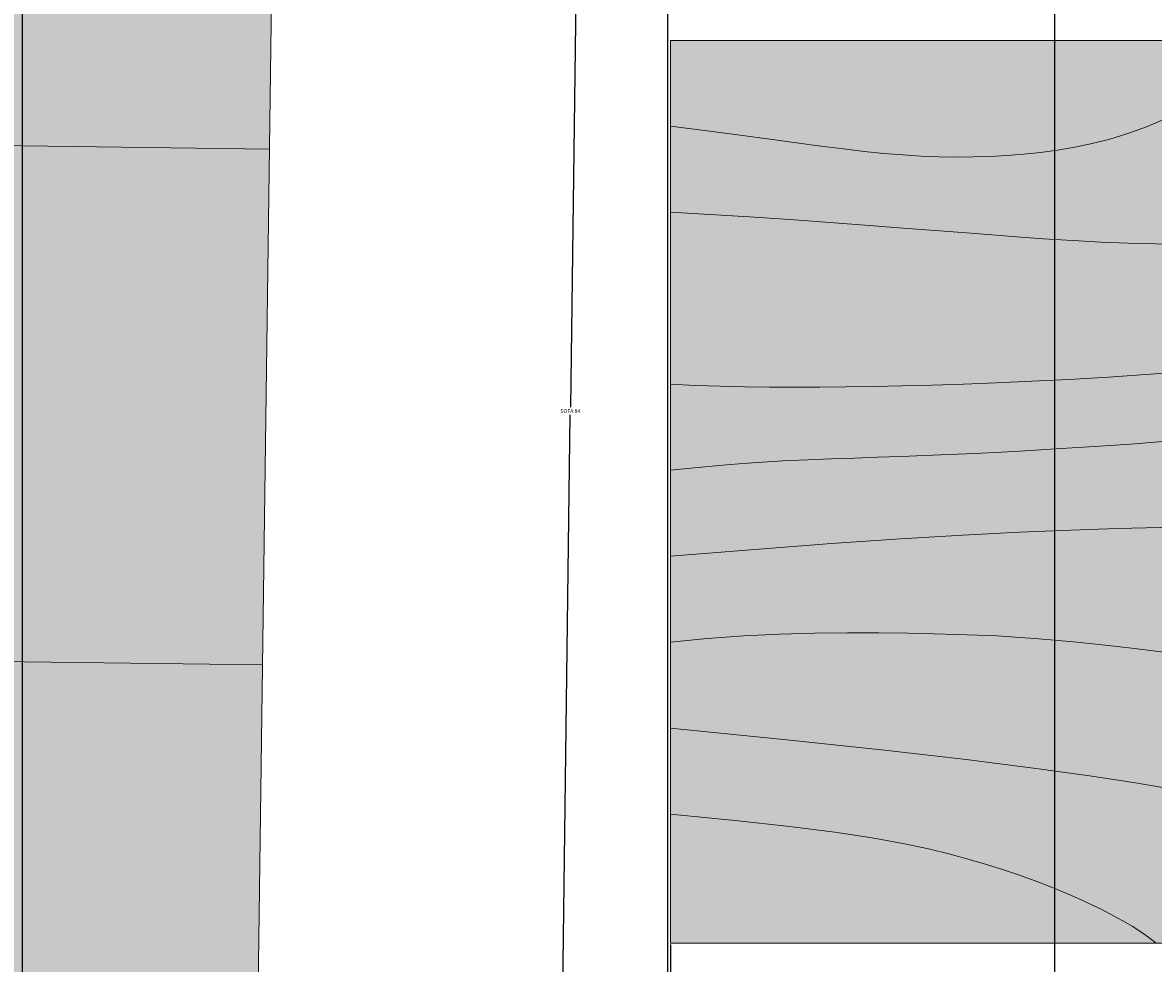
# Model space of a CAD drawing. Units: inches. Extents: x 1567 to 1964, y 1813 to 2447.
# Tile 9 of 28: x 1630 to 1683, y 2180 to 2224. Entities that reach past the tile are written whole.
import ezdxf

# ---------------------------------------------------------------- set-up
doc = ezdxf.new("R2010")
doc.units = ezdxf.units.IN
doc.layers.add('A-ANNO-DIMS', color=2, linetype='Continuous', lineweight=18)
doc.layers.add('A-FURN', color=8, linetype='Continuous', lineweight=18)
doc.layers.add('A-FURN-PATT', color=252, linetype='Continuous', lineweight=13, true_color=0x939598)
doc.styles.get("Standard").update_dxf_attribs({"font": 'arial.ttf'})
doc.dimstyles.get("Standard").update_dxf_attribs({"dimtxt": 0.18, "dimasz": 0.18, "dimexe": 0.18, "dimexo": 0.0625, "dimgap": 0.09, "dimtad": 0, "dimtih": 1, "dimtoh": 1, "dimdec": 4, "dimzin": 0, "dimdsep": 46, "dimtxsty": 'Standard', "dimcen": 0.09, "dimadec": 0, "dimazin": 0, "dimtfac": 1, "dimtdec": 4, "dimtofl": 0, "dimtmove": 0, "dimatfit": 3, "dimfxl": 1, "dimtolj": 1, "dimtzin": 0, "dimarcsym": 0})

# ---------------------------------------------------------------- blocks, each defined once
blk = doc.blocks.new('Table - Square Woodgrain 42 x 42 in.')
blk.add_line((0, -42), (42, -42))
for points in [[(0, -4), (1.704, -4.2172), (3.2358, -4.4188), (4.615, -4.604), (5.8615, -4.7721), (6.9951, -4.9224), (8.0357, -5.0541), (9.0031, -5.1667), (9.9171, -5.2594), (10.7951, -5.3316), (11.6445, -5.3836), (12.4702, -5.4157), (13.277, -5.4283), (14.0698, -5.4217), (14.8535, -5.3964), (15.6331, -5.3526), (16.4133, -5.2908), (17.1986, -5.2103), (17.9913, -5.1062), (18.793, -4.9727), (19.6056, -4.8038), (20.4307, -4.5937), (21.2701, -4.3365), (22.1256, -4.0262), (22.9989, -3.6571), (23.888, -3.2272), (24.7756, -2.7516), (25.6408, -2.2491), (26.4624, -1.7387), (27.2195, -1.2395), (27.891, -0.7703), (28.456, -0.3501), (28.8934, 0.002)], [(0, -42), (0, 0), (42, 0), (42, -42)], [(0, -8), (1.8203, -8.1001), (3.6741, -8.2149), (5.5411, -8.3408), (7.4011, -8.4741), (9.2339, -8.6112), (11.0193, -8.7484), (12.7371, -8.8821), (14.3671, -9.0086), (15.8954, -9.1246), (17.3337, -9.2278), (18.6997, -9.3159), (20.0116, -9.387), (21.2871, -9.4389), (22.5442, -9.4696), (23.8008, -9.477), (25.0749, -9.459), (26.3791, -9.4137), (27.7049, -9.3403), (29.0383, -9.2382), (30.3655, -9.1068), (31.6728, -8.9455), (32.9461, -8.7535), (34.1717, -8.5304), (35.3358, -8.2756), (36.4268, -7.9863), (37.443, -7.6521), (38.3849, -7.2603), (39.253, -6.7986), (40.048, -6.2542), (40.7705, -5.6147), (41.421, -4.8674), (42, -4)], [(42, -12), (39.1784, -12.8621), (36.4519, -13.5654), (33.8246, -14.1294), (31.3004, -14.5731), (28.8832, -14.9161), (26.577, -15.1775), (24.3858, -15.3768), (22.3136, -15.5332), (20.3622, -15.6632), (18.5254, -15.7718), (16.7947, -15.8612), (15.1618, -15.9338), (13.6183, -15.9916), (12.1558, -16.0369), (10.7659, -16.0718), (9.4403, -16.0987), (8.1703, -16.1191), (6.9461, -16.1325), (5.7577, -16.1377), (4.595, -16.1335), (3.4479, -16.1188), (2.3064, -16.0924), (1.1604, -16.0532), (0, -16)], [(42, -16), (37.6529, -16.7365), (33.8802, -17.329), (30.6179, -17.7961), (27.8015, -18.1561), (25.3668, -18.4275), (23.2497, -18.6288), (21.3859, -18.7785), (19.7111, -18.8949), (18.1693, -18.9939), (16.7375, -19.0795), (15.401, -19.1534), (14.1449, -19.217), (12.9544, -19.2717), (11.8148, -19.3191), (10.7113, -19.3606), (9.6291, -19.3976), (8.5534, -19.4323), (7.47, -19.4689), (6.3643, -19.5122), (5.222, -19.5672), (4.0288, -19.6386), (2.7703, -19.7313), (1.4321, -19.8501), (0, -20)], [(0, -24), (3.9243, -23.6805), (7.4766, -23.4138), (10.6891, -23.1954), (13.5943, -23.0205), (16.2247, -22.8847), (18.6125, -22.7832), (20.7903, -22.7116), (22.7903, -22.6651), (24.6563, -22.642), (26.4764, -22.6507), (28.35, -22.7024), (30.3766, -22.8084), (32.6555, -22.98), (35.2861, -23.2283), (38.3678, -23.5645), (42, -24)], [(42, -32), (37.392, -31.017), (33.4585, -30.2231), (30.1291, -29.5949), (27.3334, -29.109), (25.0009, -28.742), (23.0612, -28.4707), (21.4439, -28.2716), (20.0786, -28.1215), (18.8998, -28.0002), (17.8609, -27.9014), (16.9206, -27.8219), (16.0371, -27.7588), (15.1691, -27.709), (14.2748, -27.6693), (13.3128, -27.6368), (12.2415, -27.6083), (11.0295, -27.5824), (9.6867, -27.5643), (8.233, -27.5608), (6.6884, -27.5787), (5.0728, -27.6248), (3.4062, -27.7058), (1.7086, -27.8286), (0, -28)], [(0, -32), (5.4026, -32.5358), (9.9494, -33.019), (13.7424, -33.4553), (16.8834, -33.8505), (19.4743, -34.2106), (21.6171, -34.5413), (23.4136, -34.8486), (24.9657, -35.1382), (26.3614, -35.4156), (27.6332, -35.6841), (28.7995, -35.9467), (29.8788, -36.2064), (30.8897, -36.4661), (31.8507, -36.7288), (32.7802, -36.9973), (33.6968, -37.2747), (34.6175, -37.5635), (35.5531, -37.8651), (36.5128, -38.1805), (37.506, -38.5108), (38.5421, -38.8568), (39.6302, -39.2197), (40.7797, -39.6004), (42, -40)], [(0, -36), (3.0098, -36.2857), (5.5354, -36.5643), (7.6368, -36.8359), (9.374, -37.1009), (10.807, -37.3597), (11.9957, -37.6126), (13.0002, -37.8599), (13.8804, -38.102), (14.6874, -38.3393), (15.4365, -38.5729), (16.1338, -38.8041), (16.7858, -39.0341), (17.3987, -39.264), (17.9787, -39.4952), (18.5322, -39.7288), (19.0655, -39.9662), (19.5832, -40.2081), (20.0842, -40.4544), (20.5657, -40.7046), (21.0249, -40.9581), (21.459, -41.2144), (21.8653, -41.4731), (22.2409, -41.7335), (22.5831, -41.9951)]]:
    blk.add_lwpolyline(points)
blk = doc.blocks.new('Sofa - Roundback 7 ft.')
for p, q in [((-12.00002, -32.4421), (-12.00003, -6.5971)), ((11.99997, -32.4421), (11.99998, -6.5971)), ((-36.000027, -32.4421), (35.99998, -32.4421))]:
    blk.add_line(p, q)
blk = doc.blocks.new('*D23')
at = {"layer": 'A-ANNO-DIMS', "color": 0, "lineweight": -2, "transparency": 16777216}
for p, q in [((1643.923, 2247.723), (1656.64, 2247.554)), ((1656.457, 2247.376), (1655.905, 2205.743)), ((1655.347, 2163.744), (1655.9, 2205.377)), ((1642.808, 2163.73), (1655.525, 2163.561))]:
    blk.add_line(p, q, dxfattribs=at)
at = {"layer": 'A-ANNO-DIMS', "color": 0, "transparency": 16777216}
for points in [[(1656.427, 2247.377), (1656.487, 2247.376), (1656.46, 2247.556)], [(1655.317, 2163.744), (1655.377, 2163.743), (1655.345, 2163.564)]]:
    blk.add_solid(points, dxfattribs=at)
at = {"layer": 'Defpoints', "color": 0, "transparency": 16777216}
for p in [(1643.861, 2247.723), (1656.46, 2247.556), (1642.746, 2163.731)]:
    blk.add_point(p, dxfattribs=at)
at = {"layer": 'A-ANNO-DIMS', "color": 0, "transparency": 16777216, "insert": (1655.902, 2205.56), "char_height": 0.18, "attachment_point": 5}
blk.add_mtext('\\A1;SOFA 84', dxfattribs=at)
blk = doc.blocks.new('*D26')
at = {"layer": 'A-ANNO-DIMS', "color": 0, "lineweight": -2, "transparency": 16777216}
for p, q in [((1660.561, 2180.743), (1660.561, 2174.325)), ((1702.561, 2180.743), (1702.561, 2174.325)), ((1660.741, 2174.505), (1681.339, 2174.505)), ((1702.381, 2174.505), (1681.783, 2174.505))]:
    blk.add_line(p, q, dxfattribs=at)
at = {"layer": 'A-ANNO-DIMS', "color": 0, "transparency": 16777216}
for points in [[(1660.741, 2174.535), (1660.741, 2174.475), (1660.561, 2174.505)], [(1702.381, 2174.535), (1702.381, 2174.475), (1702.561, 2174.505)]]:
    blk.add_solid(points, dxfattribs=at)
at = {"layer": 'Defpoints', "color": 0, "transparency": 16777216}
for p in [(1660.561, 2180.806), (1702.561, 2180.806), (1702.561, 2174.505)]:
    blk.add_point(p, dxfattribs=at)
at = {"layer": 'A-ANNO-DIMS', "color": 0, "transparency": 16777216, "insert": (1681.561, 2174.505), "char_height": 0.18, "attachment_point": 5}
blk.add_mtext('\\A1;42', dxfattribs=at)
blk = doc.blocks.new('*D57')
at = {"layer": 'A-ANNO-DIMS', "color": 0, "lineweight": -2, "transparency": 16777216}
for p, q in [((1630.43, 2127.352), (1630.43, 2447.12)), ((1630.61, 2446.94), (1654.207, 2446.94)), ((1678.25, 2446.94), (1654.652, 2446.94)), ((1678.43, 2127.352), (1678.43, 2447.12))]:
    blk.add_line(p, q, dxfattribs=at)
at = {"layer": 'A-ANNO-DIMS', "color": 0, "transparency": 16777216}
for points in [[(1630.61, 2446.97), (1630.61, 2446.91), (1630.43, 2446.94)], [(1678.25, 2446.97), (1678.25, 2446.91), (1678.43, 2446.94)]]:
    blk.add_solid(points, dxfattribs=at)
at = {"layer": 'Defpoints', "color": 0, "transparency": 16777216}
for p in [(1678.43, 2446.94), (1630.43, 2127.29), (1678.43, 2127.29)]:
    blk.add_point(p, dxfattribs=at)
at = {"layer": 'A-ANNO-DIMS', "color": 0, "transparency": 16777216, "insert": (1654.43, 2446.94), "char_height": 0.18, "attachment_point": 5}
blk.add_mtext('\\A1;48', dxfattribs=at)
blk = doc.blocks.new('*D60')
at = {"layer": 'A-ANNO-DIMS', "color": 0, "lineweight": -2, "transparency": 16777216}
for p, q in [((1660.43, 2063.352), (1660.43, 2447.12)), ((1660.61, 2446.94), (1681.208, 2446.94)), ((1702.25, 2446.94), (1681.651, 2446.94)), ((1702.43, 2063.352), (1702.43, 2447.12))]:
    blk.add_line(p, q, dxfattribs=at)
at = {"layer": 'A-ANNO-DIMS', "color": 0, "transparency": 16777216}
for points in [[(1660.61, 2446.97), (1660.61, 2446.91), (1660.43, 2446.94)], [(1702.25, 2446.97), (1702.25, 2446.91), (1702.43, 2446.94)]]:
    blk.add_solid(points, dxfattribs=at)
at = {"layer": 'Defpoints', "color": 0, "transparency": 16777216}
for p in [(1660.43, 2446.94), (1660.43, 2063.29), (1702.43, 2063.29)]:
    blk.add_point(p, dxfattribs=at)
at = {"layer": 'A-ANNO-DIMS', "color": 0, "transparency": 16777216, "insert": (1681.43, 2446.94), "char_height": 0.18, "attachment_point": 5}
blk.add_mtext('\\A1;42', dxfattribs=at)

msp = doc.modelspace()

# ---------------------------------------------------------------- hatches: boundary and pattern name
at = {"layer": 'A-FURN-PATT'}
h = msp.add_hatch(color=256, dxfattribs=at)
h.dxf.hatch_style = 1
h.paths.add_polyline_path([(1697.3402, 2374.8316), (1682.1402, 2374.8316), (1682.1402, 2387.6316), (1637.3402, 2387.6316), (1637.3402, 2324.4315), (1697.3402, 2324.4315)])
h.paths.add_polyline_path([(1891.1093, 2375.8204), (1875.9094, 2375.8204), (1875.9094, 2388.6204), (1831.1094, 2388.6204), (1831.1094, 2325.4204), (1891.1093, 2325.4204)])
h.paths.add_polyline_path([(1702.5611, 2206.8057), (1702.5611, 2210.8057), (1699.7395, 2209.9436), (1697.013, 2209.2403), (1694.3857, 2208.6763), (1691.8615, 2208.2326), (1689.4443, 2207.8896), (1687.1381, 2207.6282), (1684.9469, 2207.4289), (1682.8747, 2207.2725), (1680.9233, 2207.1425), (1679.0865, 2207.0339), (1677.3558, 2206.9445), (1675.7229, 2206.8719), (1674.1794, 2206.8141), (1672.7169, 2206.7688), (1671.327, 2206.7339), (1670.0014, 2206.707), (1668.7314, 2206.6866), (1667.5072, 2206.6732), (1666.3188, 2206.668), (1665.1561, 2206.6722), (1664.009, 2206.6869), (1662.8675, 2206.7133), (1661.7215, 2206.7525), (1660.5611, 2206.8057), (1660.5611, 2202.8057), (1661.9932, 2202.9556), (1663.3314, 2203.0744), (1664.5899, 2203.1671), (1665.7831, 2203.2385), (1666.9254, 2203.2935), (1668.0311, 2203.3368), (1669.1145, 2203.3734), (1670.1902, 2203.4081), (1671.2724, 2203.4451), (1672.3759, 2203.4866), (1673.5155, 2203.534), (1674.706, 2203.5887), (1675.9621, 2203.6523), (1677.2986, 2203.7262), (1678.7304, 2203.8118), (1680.2722, 2203.9108), (1681.947, 2204.0272), (1683.8108, 2204.1769), (1685.9279, 2204.3782), (1688.3626, 2204.6496), (1691.179, 2205.0096), (1694.4413, 2205.4767), (1698.214, 2206.0692)])
h.paths.add_polyline_path([(1702.5611, 2218.8057), (1701.9821, 2217.9383), (1701.3316, 2217.191), (1700.6091, 2216.5515), (1699.8141, 2216.0071), (1698.946, 2215.5454), (1698.0041, 2215.1536), (1696.9879, 2214.8194), (1695.8969, 2214.5301), (1694.7328, 2214.2753), (1693.5072, 2214.0522), (1692.2339, 2213.8602), (1690.9266, 2213.6989), (1689.5994, 2213.5675), (1688.266, 2213.4654), (1686.9402, 2213.392), (1685.636, 2213.3467), (1684.3619, 2213.3287), (1683.1053, 2213.3361), (1681.8482, 2213.3668), (1680.5727, 2213.4187), (1679.2608, 2213.4898), (1677.8948, 2213.5779), (1676.4565, 2213.6811), (1674.9282, 2213.7971), (1673.2982, 2213.9236), (1671.5804, 2214.0573), (1669.795, 2214.1945), (1667.9622, 2214.3316), (1666.1022, 2214.4649), (1664.2352, 2214.5908), (1662.3814, 2214.7056), (1660.5611, 2214.8057), (1660.5611, 2206.8057), (1661.7215, 2206.7525), (1662.8675, 2206.7133), (1664.009, 2206.6869), (1665.1561, 2206.6722), (1666.3188, 2206.668), (1667.5072, 2206.6732), (1668.7314, 2206.6866), (1670.0014, 2206.707), (1671.327, 2206.7339), (1672.7169, 2206.7688), (1674.1794, 2206.8141), (1675.7229, 2206.8719), (1677.3558, 2206.9445), (1679.0865, 2207.0339), (1680.9233, 2207.1425), (1682.8747, 2207.2725), (1684.9469, 2207.4289), (1687.1381, 2207.6282), (1689.4443, 2207.8896), (1691.8615, 2208.2326), (1694.3857, 2208.6763), (1697.013, 2209.2403), (1699.7395, 2209.9436), (1702.5611, 2210.8057)])
h.paths.add_polyline_path([(1700.6091, 2216.5515), (1701.3316, 2217.191), (1701.9821, 2217.9383), (1702.5611, 2218.8057), (1702.5611, 2222.8057), (1689.452, 2222.8057), (1689.0171, 2222.4556), (1688.4521, 2222.0354), (1687.7806, 2221.5662), (1687.0235, 2221.067), (1686.2019, 2220.5566), (1685.3367, 2220.0541), (1684.4491, 2219.5785), (1683.56, 2219.1486), (1682.6867, 2218.7795), (1681.8312, 2218.4692), (1680.9918, 2218.212), (1680.1667, 2218.0019), (1679.3541, 2217.833), (1678.5524, 2217.6995), (1677.7597, 2217.5954), (1676.9744, 2217.5149), (1676.1942, 2217.4531), (1675.4146, 2217.4093), (1674.6309, 2217.384), (1673.8381, 2217.3774), (1673.0313, 2217.39), (1672.2056, 2217.4221), (1671.3562, 2217.4741), (1670.4782, 2217.5463), (1669.5642, 2217.639), (1668.5968, 2217.7516), (1667.5562, 2217.8833), (1666.4226, 2218.0336), (1665.1761, 2218.2017), (1663.7969, 2218.3869), (1662.2651, 2218.5885), (1660.5611, 2218.8057), (1660.5611, 2214.8057), (1662.3814, 2214.7056), (1664.2352, 2214.5908), (1666.1022, 2214.4649), (1667.9622, 2214.3316), (1669.795, 2214.1945), (1671.5804, 2214.0573), (1673.2982, 2213.9236), (1674.9282, 2213.7971), (1676.4565, 2213.6811), (1677.8948, 2213.5779), (1679.2608, 2213.4898), (1680.5727, 2213.4187), (1681.8482, 2213.3668), (1683.1053, 2213.3361), (1684.3619, 2213.3287), (1685.636, 2213.3467), (1686.9402, 2213.392), (1688.266, 2213.4654), (1689.5994, 2213.5675), (1690.9266, 2213.6989), (1692.2339, 2213.8602), (1693.5072, 2214.0522), (1694.7328, 2214.2753), (1695.8969, 2214.5301), (1696.9879, 2214.8194), (1698.0041, 2215.1536), (1698.946, 2215.5454), (1699.8141, 2216.0071)])
h.paths.add_polyline_path([(1687.0235, 2221.067), (1687.7806, 2221.5662), (1688.4521, 2222.0354), (1689.0171, 2222.4556), (1689.452, 2222.8057), (1660.5611, 2222.8057), (1660.5611, 2218.8057), (1662.2651, 2218.5885), (1663.7969, 2218.3869), (1665.1761, 2218.2017), (1666.4226, 2218.0336), (1667.5562, 2217.8833), (1668.5968, 2217.7516), (1669.5642, 2217.639), (1670.4782, 2217.5463), (1671.3562, 2217.4741), (1672.2056, 2217.4221), (1673.0313, 2217.39), (1673.8381, 2217.3774), (1674.6309, 2217.384), (1675.4146, 2217.4093), (1676.1942, 2217.4531), (1676.9744, 2217.5149), (1677.7597, 2217.5954), (1678.5524, 2217.6995), (1679.3541, 2217.833), (1680.1667, 2218.0019), (1680.9918, 2218.212), (1681.8312, 2218.4692), (1682.6867, 2218.7795), (1683.56, 2219.1486), (1684.4491, 2219.5785), (1685.3367, 2220.0541), (1686.2019, 2220.5566)], flags=17)
h.paths.add_polyline_path([(1702.5611, 2198.8057), (1698.9289, 2199.2412), (1695.8472, 2199.5774), (1693.2166, 2199.8257), (1690.9377, 2199.9973), (1688.9111, 2200.1033), (1687.0375, 2200.155), (1685.2174, 2200.1637), (1683.3514, 2200.1406), (1681.3514, 2200.0941), (1679.1736, 2200.0225), (1676.7858, 2199.921), (1674.1554, 2199.7852), (1671.2502, 2199.6103), (1668.0377, 2199.3919), (1664.4854, 2199.1252), (1660.5611, 2198.8057), (1660.5611, 2194.8057), (1662.2697, 2194.9771), (1663.9673, 2195.0999), (1665.6339, 2195.1809), (1667.2495, 2195.227), (1668.7941, 2195.2449), (1670.2478, 2195.2414), (1671.5906, 2195.2233), (1672.8026, 2195.1974), (1673.8739, 2195.1689), (1674.8359, 2195.1364), (1675.7302, 2195.0967), (1676.5982, 2195.0469), (1677.4817, 2194.9838), (1678.422, 2194.9043), (1679.4609, 2194.8055), (1680.6397, 2194.6842), (1682.005, 2194.5341), (1683.6223, 2194.335), (1685.562, 2194.0637), (1687.8945, 2193.6967), (1690.6902, 2193.2108), (1694.0196, 2192.5826), (1697.9531, 2191.7887), (1702.5611, 2190.8057)])
h.paths.add_polyline_path([(1702.5611, 2206.8057), (1698.214, 2206.0692), (1694.4413, 2205.4767), (1691.179, 2205.0096), (1688.3626, 2204.6496), (1685.9279, 2204.3782), (1683.8108, 2204.1769), (1681.947, 2204.0272), (1680.2722, 2203.9108), (1678.7304, 2203.8118), (1677.2986, 2203.7262), (1675.9621, 2203.6523), (1674.706, 2203.5887), (1673.5155, 2203.534), (1672.3759, 2203.4866), (1671.2724, 2203.4451), (1670.1902, 2203.4081), (1669.1145, 2203.3734), (1668.0311, 2203.3368), (1666.9254, 2203.2935), (1665.7831, 2203.2385), (1664.5899, 2203.1671), (1663.3314, 2203.0744), (1661.9932, 2202.9556), (1660.5611, 2202.8057), (1660.5611, 2198.8057), (1664.4854, 2199.1252), (1668.0377, 2199.3919), (1671.2502, 2199.6103), (1674.1554, 2199.7852), (1676.7858, 2199.921), (1679.1736, 2200.0225), (1681.3514, 2200.0941), (1683.3514, 2200.1406), (1685.2174, 2200.1637), (1687.0375, 2200.155), (1688.9111, 2200.1033), (1690.9377, 2199.9973), (1693.2166, 2199.8257), (1695.8472, 2199.5774), (1698.9289, 2199.2412), (1702.5611, 2198.8057)])
h.paths.add_polyline_path([(1702.5611, 2190.8057), (1697.9531, 2191.7887), (1694.0196, 2192.5826), (1690.6902, 2193.2108), (1687.8945, 2193.6967), (1685.562, 2194.0637), (1683.6223, 2194.335), (1682.005, 2194.5341), (1680.6397, 2194.6842), (1679.4609, 2194.8055), (1678.422, 2194.9043), (1677.4817, 2194.9838), (1676.5982, 2195.0469), (1675.7302, 2195.0967), (1674.8359, 2195.1364), (1673.8739, 2195.1689), (1672.8026, 2195.1974), (1671.5906, 2195.2233), (1670.2478, 2195.2414), (1668.7941, 2195.2449), (1667.2495, 2195.227), (1665.6339, 2195.1809), (1663.9673, 2195.0999), (1662.2697, 2194.9771), (1660.5611, 2194.8057), (1660.5611, 2190.8057), (1665.9637, 2190.2699), (1670.5105, 2189.7867), (1674.3035, 2189.3504), (1677.4445, 2188.9552), (1680.0354, 2188.5951), (1682.1782, 2188.2644), (1683.9747, 2187.9571), (1685.5268, 2187.6675), (1686.9225, 2187.3901), (1688.1943, 2187.1216), (1689.3606, 2186.859), (1690.4399, 2186.5993), (1691.4508, 2186.3396), (1692.4118, 2186.0769), (1693.3413, 2185.8084), (1694.2579, 2185.531), (1695.1786, 2185.2422), (1696.1142, 2184.9406), (1697.0739, 2184.6252), (1698.0671, 2184.2949), (1699.1032, 2183.9489), (1700.1913, 2183.586), (1701.3408, 2183.2053), (1702.5611, 2182.8057)])
h.paths.add_polyline_path([(1702.5611, 2182.8057), (1701.3408, 2183.2053), (1700.1913, 2183.586), (1699.1032, 2183.9489), (1698.0671, 2184.2949), (1697.0739, 2184.6252), (1696.1142, 2184.9406), (1695.1786, 2185.2422), (1694.2579, 2185.531), (1693.3413, 2185.8084), (1692.4118, 2186.0769), (1691.4508, 2186.3396), (1690.4399, 2186.5993), (1689.3606, 2186.859), (1688.1943, 2187.1216), (1686.9225, 2187.3901), (1685.5268, 2187.6675), (1683.9747, 2187.9571), (1682.1782, 2188.2644), (1680.0354, 2188.5951), (1677.4445, 2188.9552), (1674.3035, 2189.3504), (1670.5105, 2189.7867), (1665.9637, 2190.2699), (1660.5611, 2190.8057), (1660.5611, 2186.8057), (1663.5709, 2186.52), (1666.0965, 2186.2414), (1668.1979, 2185.9698), (1669.9351, 2185.7048), (1671.3681, 2185.446), (1672.5568, 2185.1931), (1673.5613, 2184.9458), (1674.4415, 2184.7037), (1675.2485, 2184.4664), (1675.9976, 2184.2328), (1677.0295, 2183.8907), (1678.2492, 2183.4332), (1679.354, 2182.9669), (1680.4123, 2182.4724), (1681.3757, 2181.9718), (1682.2435, 2181.4594), (1683.1864, 2180.8057), (1702.5611, 2180.8057)])
h.paths.add_polyline_path([(1677.3469, 2183.7716), (1676.6949, 2184.0016), (1675.9976, 2184.2328), (1675.2485, 2184.4664), (1674.4415, 2184.7037), (1673.5613, 2184.9458), (1672.5568, 2185.1931), (1671.3681, 2185.446), (1669.9351, 2185.7048), (1668.1979, 2185.9698), (1666.0965, 2186.2414), (1663.5709, 2186.52), (1660.5611, 2186.8057), (1660.5611, 2180.8057), (1683.1506, 2180.8057), (1682.802, 2181.0722), (1682.4264, 2181.3326), (1682.0201, 2181.5913), (1681.586, 2181.8476), (1681.1268, 2182.1011), (1680.6453, 2182.3513), (1680.1443, 2182.5976), (1679.6266, 2182.8395), (1679.0933, 2183.0769), (1678.5398, 2183.3105), (1677.9598, 2183.5417)], flags=17)
h.paths.add_polyline_path([(1824.4511, 2199.9016), (1824.089, 2199.9302), (1824.0595, 2199.9372), (1824.0397, 2199.9406), (1823.5413, 2200.0576), (1823.4095, 2200.0864), (1823.0664, 2200.1559), (1822.6419, 2200.2361), (1822.1519, 2200.3222), (1821.6126, 2200.4093), (1821.0401, 2200.4925), (1820.4505, 2200.5669), (1819.8599, 2200.6276), (1819.2845, 2200.6697), (1818.7366, 2200.6896), (1818.2141, 2200.688), (1817.7112, 2200.6668), (1817.222, 2200.6281), (1816.7405, 2200.5737), (1816.261, 2200.5057), (1815.7776, 2200.4259), (1815.2845, 2200.3364), (1814.3007, 2200.149), (1813.3315, 2199.9765), (1812.406, 2199.8514), (1811.6868, 2199.7739), (1810.8992, 2199.7121), (1810.0345, 2199.6697), (1809.0854, 2199.6497), (1808.0514, 2199.6502), (1806.9334, 2199.6683), (1805.7324, 2199.701), (1804.4493, 2199.7454), (1803.0852, 2199.7986), (1801.641, 2199.8577), (1800.1178, 2199.9197), (1798.5134, 2199.9818), (1796.8144, 2200.0415), (1795.004, 2200.0962), (1793.0657, 2200.1437), (1790.9828, 2200.1814), (1788.7389, 2200.2068), (1786.3171, 2200.2177), (1783.7011, 2200.2114), (1780.8715, 2200.185), (1777.7988, 2200.1326), (1774.4506, 2200.0481), (1770.7948, 2199.9249), (1766.7992, 2199.7569), (1762.4316, 2199.5376), (1757.6596, 2199.2606), (1752.4511, 2198.9197), (1752.4511, 2193.4197), (1761.2668, 2193.6071), (1768.3671, 2193.7934), (1773.9821, 2193.9778), (1778.3417, 2194.1593), (1781.6759, 2194.3369), (1784.2148, 2194.5096), (1786.1882, 2194.6764), (1787.8261, 2194.8364), (1789.3219, 2194.9887), (1790.7226, 2195.1333), (1792.0383, 2195.27), (1793.2792, 2195.3989), (1794.4557, 2195.52), (1795.5781, 2195.6333), (1796.6564, 2195.7387), (1797.7011, 2195.8364), (1798.7216, 2195.9259), (1799.7245, 2196.0057), (1800.7158, 2196.0737), (1801.7011, 2196.1281), (1802.6865, 2196.1668), (1803.6777, 2196.188), (1804.6806, 2196.1896), (1805.7011, 2196.1697), (1806.7423, 2196.1273), (1807.7962, 2196.0643), (1808.852, 2195.9837), (1809.899, 2195.8885), (1810.9265, 2195.7815), (1811.9238, 2195.6658), (1812.88, 2195.5442), (1813.7845, 2195.4197), (1814.6296, 2195.2948), (1815.4205, 2195.1704), (1816.1656, 2195.0469), (1816.873, 2194.9249), (1817.5511, 2194.8049), (1818.2083, 2194.6873), (1818.8527, 2194.5726), (1819.4928, 2194.4614), (1820.1348, 2194.3554), (1820.7773, 2194.2615), (1821.4169, 2194.1882), (1822.0501, 2194.1437), (1822.6735, 2194.1363), (1823.2838, 2194.1743), (1823.8775, 2194.266), (1824.4511, 2194.4197)])
h.paths.add_polyline_path([(1821.4716, 2190.5098), (1820.4303, 2190.5708), (1819.3811, 2190.6415), (1818.3339, 2190.7186), (1817.2985, 2190.7986), (1816.2845, 2190.8781), (1815.2976, 2190.9542), (1814.3274, 2191.0259), (1813.3592, 2191.0927), (1812.3782, 2191.1541), (1811.3699, 2191.2097), (1810.3196, 2191.2589), (1809.2127, 2191.3013), (1808.0345, 2191.3364), (1806.7708, 2191.3634), (1805.4094, 2191.3807), (1803.9387, 2191.3862), (1802.3469, 2191.3781), (1800.6223, 2191.3543), (1798.7532, 2191.313), (1796.7278, 2191.2521), (1794.5344, 2191.1697), (1792.128, 2191.0648), (1789.33, 2190.9393), (1785.9285, 2190.7962), (1781.7115, 2190.6385), (1776.4672, 2190.469), (1769.9836, 2190.2908), (1762.0489, 2190.1067), (1752.4511, 2189.9197), (1752.4511, 2185.4197), (1758.363, 2185.5846), (1763.4179, 2185.7075), (1767.7199, 2185.7933), (1771.373, 2185.8468), (1774.4811, 2185.873), (1777.1484, 2185.8768), (1779.4787, 2185.8629), (1781.5761, 2185.8364), (1783.5287, 2185.8014), (1785.3606, 2185.7596), (1787.0802, 2185.7119), (1788.6959, 2185.6593), (1790.2158, 2185.6028), (1791.6484, 2185.5434), (1793.0018, 2185.4821), (1794.2844, 2185.4197), (1795.5065, 2185.3576), (1796.6861, 2185.298), (1797.8433, 2185.2432), (1798.998, 2185.1958), (1800.1703, 2185.1581), (1801.3801, 2185.1326), (1802.6476, 2185.1218), (1803.9928, 2185.1281), (1805.4444, 2185.1555), (1807.0663, 2185.2147), (1808.9315, 2185.3178), (1811.1126, 2185.477), (1813.6823, 2185.7046), (1816.7135, 2186.0128), (1820.2788, 2186.4138), (1824.4511, 2186.9197), (1824.4511, 2190.4197), (1823.4918, 2190.4309), (1822.4954, 2190.4621)])
h.paths.add_polyline_path([(1797.3762, 2216.0584), (1797.6199, 2216.2267), (1797.9558, 2216.3355), (1798.3017, 2216.3703), (1798.5761, 2216.3781), (1798.8974, 2216.3703), (1799.2714, 2216.3468), (1799.704, 2216.3078), (1800.2011, 2216.2531), (1800.7695, 2216.1829), (1801.4205, 2216.0981), (1802.1662, 2215.9996), (1803.0188, 2215.8885), (1803.9906, 2215.7656), (1805.0937, 2215.632), (1806.3404, 2215.4886), (1807.7428, 2215.3364), (1809.3101, 2215.1764), (1811.039, 2215.0096), (1812.9232, 2214.8369), (1814.9563, 2214.6593), (1817.132, 2214.4778), (1819.444, 2214.2934), (1821.8858, 2214.1071), (1824.4511, 2213.9197), (1824.4511, 2217.9197), (1752.4511, 2217.9197), (1752.4511, 2214.9197), (1757.2739, 2214.8973), (1761.6432, 2214.8338), (1765.5973, 2214.7352), (1769.1751, 2214.6072), (1772.4149, 2214.4559), (1775.3554, 2214.2869), (1778.0352, 2214.1063), (1780.4928, 2213.9197), (1782.7607, 2213.7329), (1784.8476, 2213.5499), (1786.7557, 2213.3748), (1788.4876, 2213.2114), (1790.0456, 2213.0636), (1791.4322, 2212.9354), (1792.6499, 2212.8305), (1793.7011, 2212.7531), (1794.5904, 2212.7059), (1795.3313, 2212.688), (1795.9394, 2212.6974), (1796.4303, 2212.7322), (1796.8196, 2212.7905), (1797.123, 2212.8703), (1797.356, 2212.9695), (1797.5344, 2213.0864), (1797.6716, 2213.2187), (1797.7727, 2213.3637), (1797.8406, 2213.5185), (1797.8782, 2213.6801), (1797.8884, 2213.8457), (1797.8743, 2214.0122), (1797.8386, 2214.1767), (1797.7844, 2214.3364), (1797.7149, 2214.4889), (1797.6347, 2214.6346), (1797.5486, 2214.7744), (1797.3327, 2215.109), (1797.178, 2215.4303), (1797.1896, 2215.7939)])
h.paths.add_polyline_path([(1804.7872, 2210.6789), (1804.546, 2211.022), (1804.3512, 2211.3917), (1804.2466, 2211.7546), (1804.2574, 2212.0998), (1804.4058, 2212.4178), (1804.7068, 2212.7007), (1805.1359, 2212.9124), (1805.5279, 2212.9926), (1805.8136, 2213.0154), (1806.1178, 2213.0031), (1806.4405, 2212.9529), (1806.7929, 2212.867), (1807.1893, 2212.7489), (1807.6438, 2212.602), (1808.1706, 2212.4297), (1808.7838, 2212.2355), (1809.4976, 2212.0227), (1810.3261, 2211.7947), (1811.2868, 2211.5533), (1812.4101, 2211.2928), (1813.7297, 2211.0059), (1815.2793, 2210.6854), (1817.0925, 2210.3238), (1819.2031, 2209.9139), (1821.6447, 2209.4483), (1824.4511, 2208.9197), (1824.4511, 2213.9197), (1821.8858, 2214.1071), (1819.444, 2214.2934), (1817.132, 2214.4778), (1814.9563, 2214.6593), (1812.9232, 2214.8369), (1811.039, 2215.0096), (1809.3101, 2215.1764), (1807.7428, 2215.3364), (1806.3404, 2215.4886), (1805.0937, 2215.632), (1803.9906, 2215.7656), (1803.0188, 2215.8885), (1802.1662, 2215.9996), (1801.4205, 2216.0981), (1800.7695, 2216.1829), (1800.2011, 2216.2531), (1799.704, 2216.3078), (1799.2714, 2216.3468), (1798.8974, 2216.3703), (1798.5761, 2216.3781), (1798.3017, 2216.3703), (1798.0683, 2216.3468), (1797.87, 2216.3078), (1797.7011, 2216.2531), (1797.5566, 2216.1831), (1797.4355, 2216.0994), (1797.3378, 2216.004), (1797.2636, 2215.8989), (1797.2128, 2215.7859), (1797.1855, 2215.6671), (1797.1816, 2215.5444), (1797.2011, 2215.4197), (1797.2433, 2215.2946), (1797.304, 2215.1684), (1797.3783, 2215.0403), (1797.4615, 2214.9093), (1797.6718, 2214.5836), (1797.8218, 2214.2545), (1797.8933, 2213.9247), (1797.8728, 2213.5918), (1797.7366, 2213.2814), (1797.4586, 2213.0132), (1797.123, 2212.8703), (1796.8196, 2212.7905), (1796.4303, 2212.7322), (1795.9394, 2212.6974), (1795.3313, 2212.688), (1794.5904, 2212.7059), (1793.7011, 2212.7531), (1792.6499, 2212.8305), (1791.4322, 2212.9354), (1790.0456, 2213.0636), (1788.4876, 2213.2114), (1786.7557, 2213.3748), (1784.8476, 2213.5499), (1782.7607, 2213.7329), (1780.4928, 2213.9197), (1778.0352, 2214.1063), (1775.3554, 2214.2869), (1772.4149, 2214.4559), (1769.1751, 2214.6072), (1765.5973, 2214.7352), (1761.6432, 2214.8338), (1757.2739, 2214.8973), (1752.4511, 2214.9197), (1752.4511, 2209.9197), (1759.4745, 2210.0625), (1765.2786, 2210.1242), (1770.027, 2210.1175), (1773.8834, 2210.0551), (1777.0112, 2209.9498), (1779.5741, 2209.8143), (1781.7357, 2209.6611), (1783.6594, 2209.5031), (1785.4813, 2209.3506), (1787.2265, 2209.2049), (1788.8926, 2209.0651), (1790.4771, 2208.9301), (1791.9777, 2208.7991), (1793.3919, 2208.671), (1794.7171, 2208.5449), (1795.9511, 2208.4197), (1797.0922, 2208.2952), (1798.1425, 2208.1736), (1799.1049, 2208.0579), (1799.9823, 2207.951), (1800.7778, 2207.8558), (1801.4941, 2207.7752), (1802.1342, 2207.7122), (1802.7011, 2207.6697), (1803.1982, 2207.65), (1803.6308, 2207.6528), (1804.0048, 2207.6771), (1804.3261, 2207.7218), (1804.6005, 2207.7861), (1804.8339, 2207.869), (1805.0322, 2207.9694), (1805.2011, 2208.0864), (1805.3455, 2208.2189), (1805.4654, 2208.365), (1805.56, 2208.5229), (1805.6282, 2208.6906), (1805.6691, 2208.866), (1805.6816, 2209.0473), (1805.6648, 2209.2326), (1805.6178, 2209.4197), (1805.5406, 2209.6072), (1805.4381, 2209.7947), (1805.316, 2209.9822), (1805.1803, 2210.1697), (1805.0367, 2210.3572)])
h.paths.add_polyline_path([(1801.4941, 2207.7752), (1800.7778, 2207.8558), (1799.9823, 2207.951), (1799.1049, 2208.0579), (1798.1425, 2208.1736), (1797.0922, 2208.2952), (1795.9511, 2208.4197), (1794.7171, 2208.5449), (1793.3919, 2208.671), (1791.9777, 2208.7991), (1790.4771, 2208.9301), (1788.8926, 2209.0651), (1787.2265, 2209.2049), (1785.4813, 2209.3506), (1783.6594, 2209.5031), (1781.7357, 2209.6611), (1779.5741, 2209.8143), (1777.0112, 2209.9498), (1773.8834, 2210.0551), (1770.027, 2210.1175), (1765.2786, 2210.1242), (1759.4745, 2210.0625), (1752.4511, 2209.9197), (1752.4511, 2205.4197), (1757.7354, 2205.2545), (1762.3821, 2205.1294), (1766.4565, 2205.0374), (1770.024, 2204.9718), (1773.1502, 2204.9258), (1775.9003, 2204.8924), (1778.3399, 2204.8649), (1780.5344, 2204.8364), (1782.5421, 2204.8014), (1784.3925, 2204.7596), (1786.1082, 2204.7119), (1787.7115, 2204.6593), (1789.225, 2204.6028), (1790.6711, 2204.5434), (1792.0724, 2204.4821), (1793.4511, 2204.4197), (1794.8241, 2204.3576), (1796.1855, 2204.2973), (1797.5234, 2204.241), (1798.8261, 2204.1906), (1800.082, 2204.1479), (1801.2792, 2204.115), (1802.4062, 2204.0939), (1803.4511, 2204.0864), (1804.4051, 2204.0942), (1805.2701, 2204.1176), (1806.0512, 2204.1567), (1806.7532, 2204.2114), (1807.381, 2204.2817), (1807.9394, 2204.3676), (1808.4334, 2204.4692), (1808.8678, 2204.5864), (1809.248, 2204.7187), (1809.5813, 2204.8637), (1809.8756, 2205.0185), (1810.1386, 2205.1801), (1810.3782, 2205.3457), (1810.6022, 2205.5122), (1810.9725, 2205.7941), (1811.3803, 2206.072), (1811.739, 2206.2612), (1812.0032, 2206.3781), (1812.2869, 2206.4793), (1812.5931, 2206.563), (1812.9246, 2206.6271), (1813.2845, 2206.6697), (1813.6746, 2206.6894), (1814.0931, 2206.6867), (1814.5369, 2206.6624), (1815.0032, 2206.6176), (1815.489, 2206.5534), (1815.9915, 2206.4705), (1816.5076, 2206.3701), (1817.0345, 2206.2531), (1817.5753, 2206.1196), (1818.1582, 2205.9666), (1818.8172, 2205.7902), (1819.5865, 2205.5864), (1820.5004, 2205.3514), (1821.5931, 2205.0812), (1822.8986, 2204.7719), (1824.4511, 2204.4197), (1824.4511, 2208.9197), (1821.6447, 2209.4483), (1819.2031, 2209.9139), (1817.0925, 2210.3238), (1815.2793, 2210.6854), (1813.7297, 2211.0059), (1812.4101, 2211.2928), (1811.2868, 2211.5533), (1810.3261, 2211.7947), (1809.4976, 2212.0227), (1808.7838, 2212.2355), (1808.1706, 2212.4297), (1807.6438, 2212.602), (1807.1893, 2212.7489), (1806.7929, 2212.867), (1806.4405, 2212.9529), (1806.1178, 2213.0031), (1805.8136, 2213.0154), (1805.5279, 2212.9926), (1805.2638, 2212.9386), (1805.024, 2212.8572), (1804.8116, 2212.7524), (1804.6295, 2212.6281), (1804.4806, 2212.4881), (1804.3678, 2212.3364), (1804.2931, 2212.1764), (1804.2545, 2212.0096), (1804.2491, 2211.8369), (1804.274, 2211.6593), (1804.3263, 2211.4778), (1804.4029, 2211.2934), (1804.5011, 2211.1071), (1804.6178, 2210.9197), (1804.7496, 2210.7322), (1804.8912, 2210.5447), (1805.154, 2210.2061), (1805.3962, 2209.8715), (1805.5964, 2209.5053), (1805.688, 2209.1402), (1805.6629, 2208.7758), (1805.5257, 2208.4385), (1805.2839, 2208.1437), (1804.9434, 2207.9078), (1804.6005, 2207.7861), (1804.3261, 2207.7218), (1804.0048, 2207.6771), (1803.6308, 2207.6528), (1803.1982, 2207.65), (1802.7011, 2207.6697), (1802.1342, 2207.7122)])
h.paths.add_polyline_path([(1824.4511, 2204.4197), (1822.8986, 2204.7719), (1821.5931, 2205.0812), (1820.5004, 2205.3514), (1819.5865, 2205.5864), (1818.8172, 2205.7902), (1818.1582, 2205.9666), (1817.5753, 2206.1196), (1817.0345, 2206.2531), (1816.5076, 2206.3701), (1815.9915, 2206.4705), (1815.489, 2206.5534), (1815.0032, 2206.6176), (1814.5369, 2206.6624), (1814.0931, 2206.6867), (1813.6746, 2206.6894), (1813.2845, 2206.6697), (1812.9246, 2206.6271), (1812.5931, 2206.563), (1812.2869, 2206.4793), (1812.0032, 2206.3781), (1811.739, 2206.2612), (1811.4915, 2206.1307), (1811.2576, 2205.9884), (1811.0345, 2205.8364), (1810.8183, 2205.6767), (1810.4357, 2205.3854), (1810.1386, 2205.1801), (1809.8756, 2205.0185), (1809.5813, 2204.8637), (1809.248, 2204.7187), (1808.8678, 2204.5864), (1808.4334, 2204.4692), (1807.9394, 2204.3676), (1807.381, 2204.2817), (1806.7532, 2204.2114), (1806.0512, 2204.1567), (1805.2701, 2204.1176), (1804.4051, 2204.0942), (1803.4511, 2204.0864), (1802.4062, 2204.0939), (1801.2792, 2204.115), (1800.082, 2204.1479), (1798.8261, 2204.1906), (1797.5234, 2204.241), (1796.1855, 2204.2973), (1794.8241, 2204.3576), (1793.4511, 2204.4197), (1792.0724, 2204.4821), (1790.6711, 2204.5434), (1789.225, 2204.6028), (1787.7115, 2204.6593), (1786.1082, 2204.7119), (1784.3925, 2204.7596), (1782.5421, 2204.8014), (1780.5344, 2204.8364), (1778.3399, 2204.8649), (1775.9003, 2204.8924), (1773.1502, 2204.9258), (1770.024, 2204.9718), (1766.4565, 2205.0374), (1762.3821, 2205.1294), (1757.7354, 2205.2545), (1752.4511, 2205.4197), (1752.4511, 2198.9197), (1757.6596, 2199.2606), (1762.4316, 2199.5376), (1766.7992, 2199.7569), (1770.7948, 2199.9249), (1774.4506, 2200.0481), (1777.7988, 2200.1326), (1780.8715, 2200.185), (1783.7011, 2200.2114), (1786.3171, 2200.2177), (1788.7389, 2200.2068), (1790.9828, 2200.1814), (1793.0657, 2200.1437), (1795.004, 2200.0962), (1796.8144, 2200.0415), (1798.5134, 2199.9818), (1800.1178, 2199.9197), (1801.641, 2199.8577), (1803.0852, 2199.7986), (1804.4493, 2199.7454), (1805.7324, 2199.701), (1806.9334, 2199.6683), (1808.0514, 2199.6502), (1809.0854, 2199.6497), (1810.0345, 2199.6697), (1810.8992, 2199.7121), (1811.6868, 2199.7739), (1812.406, 2199.8514), (1813.0657, 2199.9406), (1813.6746, 2200.0376), (1814.2415, 2200.1385), (1814.7752, 2200.2394), (1815.2845, 2200.3364), (1815.7776, 2200.4259), (1816.261, 2200.5057), (1816.7405, 2200.5737), (1817.222, 2200.6281), (1817.7112, 2200.6668), (1818.2141, 2200.688), (1818.7366, 2200.6896), (1819.2845, 2200.6697), (1819.8599, 2200.6276), (1820.4505, 2200.5669), (1821.0401, 2200.4925), (1821.6126, 2200.4093), (1822.1519, 2200.3222), (1822.6419, 2200.2361), (1823.0664, 2200.1559), (1823.5408, 2200.0598), (1824.0595, 2199.9372), (1824.1105, 2199.9285), (1824.1888, 2199.9223), (1824.2953, 2199.9201), (1824.4511, 2199.9197)])
h.paths.add_polyline_path([(1795.4295, 2021.5492), (1771.4295, 2021.5492), (1771.4295, 1988.29), (1735.4295, 1988.29), (1735.4295, 2055.79), (1711.4295, 2055.79), (1711.4295, 1964.29), (1795.4295, 1964.29)])
h.paths.add_polyline_path([(1681.4295, 2063.29), (1674.0411, 2043.4455), (1681.4295, 2043.4455), (1688.818, 2043.4455)])
h.paths.add_polyline_path([(1843.2327, 2065.967), (1919.26, 2065.967), (1919.26, 2095.8187), (1843.2327, 2095.8187)], flags=9)
h = msp.add_hatch(color=256, dxfattribs=at)
h.dxf.hatch_style = 1
h.paths.add_polyline_path([(1642.2233, 2241.7446), (1623.1648, 2241.9976), (1622.8462, 2217.9997), (1641.9047, 2217.7467)])
h.paths.add_polyline_path([(1641.9047, 2217.7467), (1622.8462, 2217.9997), (1622.5277, 2194.0018), (1641.5862, 2193.7488)])
h.paths.add_polyline_path([(1641.5862, 2193.7488), (1622.5277, 2194.0018), (1622.2091, 2170.0039), (1641.2677, 2169.7509)])
h.paths.add_polyline_path([(1671.2154, 2243.8726, -0.236068), (1673.5306, 2245.0302), (1673.5306, 2246.1879), (1653.8509, 2246.1879), (1653.8509, 2245.0302, -0.236068), (1656.1662, 2243.8726), (1656.1662, 2233.4539, -0.236068), (1653.8509, 2232.2963), (1653.8509, 2231.1387, 0.1176471), (1673.5306, 2231.1387), (1673.5306, 2232.2963, -0.236068), (1671.2154, 2233.4539)])
h.paths.add_polyline_path([(1703.7736, 2243.8726, -0.236068), (1706.0889, 2245.0302), (1706.0889, 2246.1879), (1686.4092, 2246.1879), (1686.4092, 2245.0302, -0.236068), (1688.7245, 2243.8726), (1688.7245, 2233.4539, -0.236068), (1686.4092, 2232.2963), (1686.4092, 2231.1387, 0.1176471), (1706.0889, 2231.1387), (1706.0889, 2232.2963, -0.236068), (1703.7736, 2233.4539)])
h.paths.add_polyline_path([(1782.6855, 2225.9197), (1766.2168, 2225.9197), (1764.9668, 2217.9197), (1783.9356, 2217.9197)])
h.paths.add_polyline_path([(1810.6855, 2225.9197), (1794.2168, 2225.9197), (1792.9668, 2217.9197), (1811.9356, 2217.9197)])
h.paths.add_polyline_path([(1752.4511, 2209.4041), (1744.4511, 2208.1541), (1744.4511, 2191.6853), (1752.4511, 2190.4354)])
h.paths.add_polyline_path([(1783.9356, 2181.9197), (1764.9668, 2181.9197), (1766.2168, 2173.9197), (1782.6855, 2173.9197)])
h.paths.add_polyline_path([(1811.9356, 2181.9197), (1792.9668, 2181.9197), (1794.2168, 2173.9197), (1810.6855, 2173.9197)])
h.paths.add_polyline_path([(1832.4511, 2208.1541), (1824.4511, 2209.4041), (1824.4511, 2190.4354), (1832.4511, 2191.6853)])
h.paths.add_polyline_path([(1824.4511, 2194.4197), (1823.8775, 2194.266), (1823.2838, 2194.1743), (1822.6735, 2194.1363), (1822.0501, 2194.1437), (1821.4169, 2194.1882), (1820.7773, 2194.2615), (1820.1348, 2194.3554), (1819.4928, 2194.4614), (1818.8527, 2194.5726), (1818.2083, 2194.6873), (1817.5511, 2194.8049), (1816.873, 2194.9249), (1816.1656, 2195.0469), (1815.4205, 2195.1704), (1814.6296, 2195.2948), (1813.7845, 2195.4197), (1812.88, 2195.5442), (1811.9238, 2195.6658), (1810.9265, 2195.7815), (1809.899, 2195.8885), (1808.852, 2195.9837), (1807.7962, 2196.0643), (1806.7423, 2196.1273), (1805.7011, 2196.1697), (1804.6806, 2196.1896), (1803.6777, 2196.188), (1802.6865, 2196.1668), (1801.7011, 2196.1281), (1800.7158, 2196.0737), (1799.7245, 2196.0057), (1798.7216, 2195.9259), (1797.7011, 2195.8364), (1796.6564, 2195.7387), (1795.5781, 2195.6333), (1794.4557, 2195.52), (1793.2792, 2195.3989), (1792.0383, 2195.27), (1790.7226, 2195.1333), (1789.3219, 2194.9887), (1787.8261, 2194.8364), (1786.1882, 2194.6764), (1784.2148, 2194.5096), (1781.6759, 2194.3369), (1778.3417, 2194.1593), (1773.9821, 2193.9778), (1768.3671, 2193.7934), (1761.2668, 2193.6071), (1752.4511, 2193.4197), (1752.4511, 2189.9197), (1762.0489, 2190.1067), (1769.9836, 2190.2908), (1776.4672, 2190.469), (1781.7115, 2190.6385), (1785.9285, 2190.7962), (1789.33, 2190.9393), (1792.128, 2191.0648), (1794.5344, 2191.1697), (1796.7278, 2191.2521), (1798.7532, 2191.313), (1800.6223, 2191.3543), (1802.3469, 2191.3781), (1803.9387, 2191.3862), (1805.4094, 2191.3807), (1806.7708, 2191.3634), (1808.0345, 2191.3364), (1809.2127, 2191.3013), (1810.3196, 2191.2589), (1811.3699, 2191.2097), (1812.3782, 2191.1541), (1813.3592, 2191.0927), (1814.3274, 2191.0259), (1815.2976, 2190.9542), (1816.2845, 2190.8781), (1817.2985, 2190.7986), (1818.3339, 2190.7186), (1819.3811, 2190.6415), (1820.4303, 2190.5708), (1821.4716, 2190.5098), (1822.4954, 2190.4621), (1823.4918, 2190.4309), (1824.3581, 2190.4208), (1824.4511, 2190.4354)])
h.paths.add_polyline_path([(1874.6531, 1991.3071), (1861.053, 1991.3071), (1859.053, 1993.3071), (1853.8531, 1993.3071), (1853.8531, 1978.1071), (1874.6531, 1978.1071)], flags=17)
h.paths.add_polyline_path([(1897.8531, 1991.3071), (1877.0531, 1991.3071), (1877.0531, 1978.1071), (1897.8531, 1978.1071)], flags=17)
h.paths.add_polyline_path([(1853.8531, 1993.3071), (1859.053, 1993.3071), (1845.8531, 2006.5071), (1845.8531, 1976.9071), (1905.853, 1976.9071), (1905.853, 1991.3071), (1897.8531, 1991.3071), (1897.8531, 1978.1071), (1877.0531, 1978.1071), (1877.0531, 1991.3071), (1874.6531, 1991.3071), (1874.6531, 1978.1071), (1853.8531, 1978.1071)])
h.paths.add_polyline_path([(1920.7245, 2259.29), (1899.7245, 2259.29), (1899.7245, 2251.29), (1920.7245, 2251.29)])
h.paths.add_polyline_path([(1918.7245, 2252.29, 0.5000001), (1919.7245, 2253.29), (1919.7245, 2257.29, 0.5000001), (1918.7245, 2258.29), (1901.7245, 2258.29, 0.5000001), (1900.7245, 2257.29), (1900.7245, 2253.29, 0.5000001), (1901.7245, 2252.29)], flags=16)
h.paths.add_polyline_path([(1843.2327, 2065.967), (1919.26, 2065.967), (1919.26, 2095.8187), (1843.2327, 2095.8187)], flags=9)

# ---------------------------------------------------------------- block references
at = {"layer": 'A-FURN', "rotation": 89.2395118843373}
msp.add_blockref('Sofa - Roundback 7 ft.', (1609.3062, 2206.1784), dxfattribs=at)
at = {"layer": 'A-FURN'}
msp.add_blockref('Table - Square Woodgrain 42 x 42 in.', (1660.5611, 2222.8057), dxfattribs=at)

# ---------------------------------------------------------------- dimensions: what is measured, and where the dimension line sits
at = {"layer": 'A-ANNO-DIMS'}
for base, p1, p2, picture, middle in [((1678.4295, 2446.94), (1630.4295, 2127.29), (1678.4295, 2127.29), '*D57', (1654.4295, 2446.94)), ((1660.4295, 2446.94), (1702.4295, 2063.29), (1660.4295, 2063.29), '*D60', (1681.4295, 2446.94)), ((1702.5611, 2174.5054), (1660.5611, 2180.8057), (1702.5611, 2180.8057), '*D26', (1681.5611, 2174.5054))]:
    dim = msp.add_linear_dim(base=base, p1=p1, p2=p2, dimstyle='Standard', override={"dimdec": 0, "dimlfac": 1, "dimrnd": 0, "dimzin": 0, "dimdsep": 46, "dimlunit": 2}, dxfattribs=at)
    dim.commit()
    dim.dimension.update_dxf_attribs({"geometry": picture, "text_midpoint": middle})
dim = msp.add_linear_dim(base=(1656.4596, 2247.5562), p1=(1642.7458, 2163.7308), p2=(1643.8607, 2247.7234), angle=89.23951, text='SOFA <>', dimstyle='Standard', override={"dimdec": 0, "dimlfac": 1, "dimrnd": 0, "dimzin": 0, "dimdsep": 46, "dimlunit": 2}, dxfattribs=at)
dim.commit()
dim.dimension.update_dxf_attribs({"geometry": '*D23', "text_midpoint": (1655.9021, 2205.5598)})

doc.saveas('drawing.dxf')
